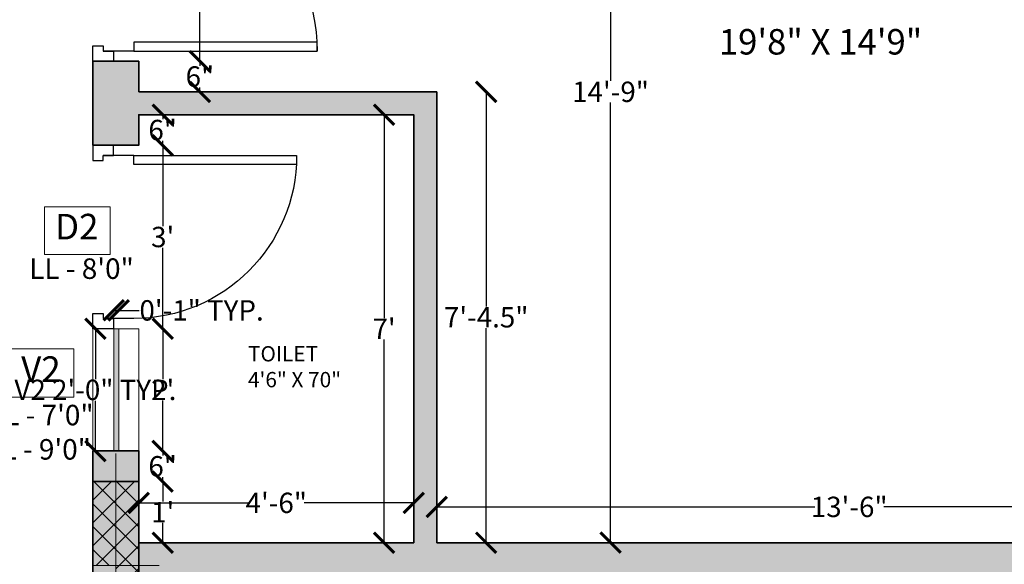
# Model space of a CAD drawing. Units: inches. Extents: x 2 to 905, y 9 to 678.
# Tile 4 of 8: x 102 to 295, y 367 to 474. Entities that reach past the tile are written whole.
import ezdxf

# ---------------------------------------------------------------- set-up
doc = ezdxf.new("R2010")
doc.units = ezdxf.units.IN
doc.linetypes.add('ACAD_ISO02W100', pattern=[15, 12, -3])
for name, color, linetype, lineweight in [('A-ANNO-DIMS', 7, 'Continuous', 18), ('A-COLS', 1, 'Continuous', 35), ('A-COLS-MARK', 1, 'Continuous', 18), ('A-COLS-PATT', 1, 'Continuous', 13), ('A-DOOR', 7, 'Continuous', 25), ('A-GLAZ', 4, 'Continuous', 18), ('A-WALL', 7, 'Continuous', 35), ('A-WALL-HIDN', 7, 'ACAD_ISO02W100', 18)]:
    doc.layers.add(name, color=color, linetype=linetype, lineweight=lineweight)
for name, color, linetype, lineweight, true_color in [('A-ANNO-IDEN', 251, 'Continuous', 18, 0x636466), ('A-AREA-IDEN', 252, 'Continuous', 18, 0x989898), ('A-WALL-PATT', 252, 'Continuous', 13, 0x939598)]:
    doc.layers.add(name, color=color, linetype=linetype, lineweight=lineweight, true_color=true_color)
doc.styles.add('PDF ArialMT', font='arial.ttf')
doc.styles.add('PDF Century Gothic Bold', font='txt')
doc.styles.get("Standard").update_dxf_attribs({"font": 'arial.ttf'})
doc.dimstyles.get("Standard").update_dxf_attribs({"dimtxt": 4, "dimasz": 4, "dimexe": 0.18, "dimexo": 0.0625, "dimgap": 0.09, "dimtad": 0, "dimtih": 1, "dimtoh": 1, "dimdec": 1, "dimzin": 0, "dimdsep": 46, "dimlunit": 3, "dimtxsty": 'Standard', "dimblk": 'ARCHTICK', "dimcen": 0, "dimse1": 1, "dimse2": 1, "dimclrt": 1, "dimadec": 0, "dimazin": 0, "dimtfac": 1, "dimtdec": 1, "dimtofl": 0, "dimtmove": 0, "dimatfit": 3, "dimfxl": 1, "dimtolj": 1, "dimtzin": 0, "dimarcsym": 0})

# ---------------------------------------------------------------- blocks, each defined once
blk = doc.blocks.new('*U4')
for p, q in [((0, 0), (0, -6)), ((-32, 0), (-32, -6))]:
    blk.add_line(p, q)
blk.add_lwpolyline([(0, 0), (0, 32), (-1.75, 32), (-1.75, 0)], close=True)
blk.add_arc((0, 0), 32, 90, 180)
blk = doc.blocks.new('*U5')
for p, q in [((0, 0), (0, -6)), ((36, 0), (36, -6))]:
    blk.add_line(p, q)
blk.add_lwpolyline([(0, 0), (0, 36), (1.75, 36), (1.75, 0)], close=True)
blk.add_arc((0, 0), 36, 0, 90)
blk = doc.blocks.new('_ArchTick')
at = {"color": 0, "linetype": 'ByBlock', "const_width": 0.15}
blk.add_lwpolyline([(-0.5, -0.5), (0.5, 0.5)], dxfattribs=at)
blk = doc.blocks.new('*D11')
at = {"layer": 'A-ANNO-DIMS', "color": 0, "lineweight": -2, "transparency": 16777216}
for p, q in [((218.07, 548.58), (218.07, 462.21)), ((218.07, 371.58), (218.07, 457.95))]:
    blk.add_line(p, q, dxfattribs=at)
at = {"layer": 'Defpoints', "color": 0, "transparency": 16777216}
for p in [(360.93, 548.58), (218.07, 371.58), (360.93, 371.58)]:
    blk.add_point(p, dxfattribs=at)
at = {"layer": 'A-ANNO-DIMS', "color": 0, "lineweight": -2, "transparency": 16777216, "xscale": 4, "yscale": 4, "zscale": 4}
for p, rotation in [((218.07, 548.58), 90), ((218.07, 371.58), 270)]:
    blk.add_blockref('_ArchTick', p, dxfattribs=dict(at, rotation=rotation))
at = {"layer": 'A-ANNO-DIMS', "color": 0, "transparency": 16777216, "insert": (218.07, 460.08), "char_height": 4, "attachment_point": 5}
blk.add_mtext('\\A1;14\'-9"', dxfattribs=at)
blk = doc.blocks.new('*D48')
at = {"layer": 'A-ANNO-DIMS', "color": 0, "lineweight": -2, "transparency": 16777216}
for p, q in [((130.12, 383.58), (130.12, 379.68)), ((130.12, 371.58), (130.12, 375.48))]:
    blk.add_line(p, q, dxfattribs=at)
at = {"layer": 'Defpoints', "color": 0, "transparency": 16777216}
for p in [(125.43, 383.58), (130.12, 383.58), (125.43, 371.58)]:
    blk.add_point(p, dxfattribs=at)
at = {"layer": 'A-ANNO-DIMS', "color": 0, "lineweight": -2, "transparency": 16777216, "xscale": 4, "yscale": 4, "zscale": 4}
for p, rotation in [((130.12, 383.58), 90), ((130.12, 371.58), 270)]:
    blk.add_blockref('_ArchTick', p, dxfattribs=dict(at, rotation=rotation))
at = {"layer": 'A-ANNO-DIMS', "color": 0, "transparency": 16777216, "insert": (130.12, 377.58), "char_height": 4, "attachment_point": 5}
blk.add_mtext("\\A1;1'", dxfattribs=at)
blk = doc.blocks.new('*D49')
at = {"layer": 'A-ANNO-DIMS', "color": 0, "lineweight": -2, "transparency": 16777216}
for p, q in [((130.12, 389.58), (130.12, 388.71)), ((130.12, 383.58), (130.12, 384.45))]:
    blk.add_line(p, q, dxfattribs=at)
at = {"layer": 'Defpoints', "color": 0, "transparency": 16777216}
for p in [(125.43, 389.58), (130.12, 389.58), (125.43, 383.58)]:
    blk.add_point(p, dxfattribs=at)
at = {"layer": 'A-ANNO-DIMS', "color": 0, "lineweight": -2, "transparency": 16777216, "xscale": 4, "yscale": 4, "zscale": 4}
for p, rotation in [((130.12, 389.58), 90), ((130.12, 383.58), 270)]:
    blk.add_blockref('_ArchTick', p, dxfattribs=dict(at, rotation=rotation))
at = {"layer": 'A-ANNO-DIMS', "color": 0, "transparency": 16777216, "insert": (130.12, 386.58), "char_height": 4, "attachment_point": 5}
blk.add_mtext('\\A1;6"', dxfattribs=at)
blk = doc.blocks.new('*D50')
at = {"layer": 'A-ANNO-DIMS', "color": 0, "lineweight": -2, "transparency": 16777216}
for p, q in [((130.12, 413.58), (130.12, 403.68)), ((130.12, 389.58), (130.12, 399.48))]:
    blk.add_line(p, q, dxfattribs=at)
at = {"layer": 'Defpoints', "color": 0, "transparency": 16777216}
for p in [(125.43, 413.58), (130.12, 413.58), (125.43, 389.58)]:
    blk.add_point(p, dxfattribs=at)
at = {"layer": 'A-ANNO-DIMS', "color": 0, "lineweight": -2, "transparency": 16777216, "xscale": 4, "yscale": 4, "zscale": 4}
for p, rotation in [((130.12, 413.58), 90), ((130.12, 389.58), 270)]:
    blk.add_blockref('_ArchTick', p, dxfattribs=dict(at, rotation=rotation))
at = {"layer": 'A-ANNO-DIMS', "color": 0, "transparency": 16777216, "insert": (130.12, 401.58), "char_height": 4, "attachment_point": 5}
blk.add_mtext("\\A1;2'", dxfattribs=at)
blk = doc.blocks.new('*D51')
at = {"layer": 'A-ANNO-DIMS', "color": 0, "lineweight": -2, "transparency": 16777216}
for p, q in [((130.12, 449.58), (130.12, 433.71)), ((130.12, 413.58), (130.12, 429.44))]:
    blk.add_line(p, q, dxfattribs=at)
at = {"layer": 'Defpoints', "color": 0, "transparency": 16777216}
for p in [(125.43, 449.58), (130.12, 449.58), (125.43, 413.58)]:
    blk.add_point(p, dxfattribs=at)
at = {"layer": 'A-ANNO-DIMS', "color": 0, "lineweight": -2, "transparency": 16777216, "xscale": 4, "yscale": 4, "zscale": 4}
for p, rotation in [((130.12, 449.58), 90), ((130.12, 413.58), 270)]:
    blk.add_blockref('_ArchTick', p, dxfattribs=dict(at, rotation=rotation))
at = {"layer": 'A-ANNO-DIMS', "color": 0, "transparency": 16777216, "insert": (130.12, 431.58), "char_height": 4, "attachment_point": 5}
blk.add_mtext("\\A1;3'", dxfattribs=at)
blk = doc.blocks.new('*D52')
at = {"layer": 'A-ANNO-DIMS', "color": 0, "lineweight": -2, "transparency": 16777216}
for p, q in [((130.12, 455.58), (130.12, 454.71)), ((130.12, 449.58), (130.12, 450.45))]:
    blk.add_line(p, q, dxfattribs=at)
at = {"layer": 'Defpoints', "color": 0, "transparency": 16777216}
for p in [(125.43, 455.58), (130.12, 455.58), (125.43, 449.58)]:
    blk.add_point(p, dxfattribs=at)
at = {"layer": 'A-ANNO-DIMS', "color": 0, "lineweight": -2, "transparency": 16777216, "xscale": 4, "yscale": 4, "zscale": 4}
for p, rotation in [((130.12, 455.58), 90), ((130.12, 449.58), 270)]:
    blk.add_blockref('_ArchTick', p, dxfattribs=dict(at, rotation=rotation))
at = {"layer": 'A-ANNO-DIMS', "color": 0, "transparency": 16777216, "insert": (130.12, 452.58), "char_height": 4, "attachment_point": 5}
blk.add_mtext('\\A1;6"', dxfattribs=at)
blk = doc.blocks.new('*D53')
at = {"layer": 'A-ANNO-DIMS', "color": 0, "lineweight": -2, "transparency": 16777216}
for p, q in [((137.43, 466.08), (137.43, 465.21)), ((137.43, 460.08), (137.43, 460.95))]:
    blk.add_line(p, q, dxfattribs=at)
at = {"layer": 'Defpoints', "color": 0, "transparency": 16777216}
for p in [(132.75, 466.08), (137.43, 466.08), (132.75, 460.08)]:
    blk.add_point(p, dxfattribs=at)
at = {"layer": 'A-ANNO-DIMS', "color": 0, "lineweight": -2, "transparency": 16777216, "xscale": 4, "yscale": 4, "zscale": 4}
for p, rotation in [((137.43, 466.08), 90), ((137.43, 460.08), 270)]:
    blk.add_blockref('_ArchTick', p, dxfattribs=dict(at, rotation=rotation))
at = {"layer": 'A-ANNO-DIMS', "color": 0, "transparency": 16777216, "insert": (137.43, 463.08), "char_height": 4, "attachment_point": 5}
blk.add_mtext('\\A1;6"', dxfattribs=at)
blk = doc.blocks.new('*D54')
at = {"layer": 'A-ANNO-DIMS', "color": 0, "lineweight": -2, "transparency": 16777216}
for p, q in [((137.43, 506.08), (137.43, 488.21)), ((137.43, 466.08), (137.43, 483.94))]:
    blk.add_line(p, q, dxfattribs=at)
at = {"layer": 'Defpoints', "color": 0, "transparency": 16777216}
for p in [(132.75, 506.08), (137.43, 506.08), (132.75, 466.08)]:
    blk.add_point(p, dxfattribs=at)
at = {"layer": 'A-ANNO-DIMS', "color": 0, "lineweight": -2, "transparency": 16777216, "xscale": 4, "yscale": 4, "zscale": 4}
for p, rotation in [((137.43, 506.08), 90), ((137.43, 466.08), 270)]:
    blk.add_blockref('_ArchTick', p, dxfattribs=dict(at, rotation=rotation))
at = {"layer": 'A-ANNO-DIMS', "color": 0, "transparency": 16777216, "insert": (137.43, 486.08), "char_height": 4, "attachment_point": 5}
blk.add_mtext('\\A1;3\'-4"', dxfattribs=at)
blk = doc.blocks.new('*D65')
at = {"layer": 'A-ANNO-DIMS', "color": 0, "lineweight": -2, "transparency": 16777216}
for p, q in [((183.93, 378.61), (258.16, 378.61)), ((345.93, 378.61), (271.71, 378.61))]:
    blk.add_line(p, q, dxfattribs=at)
at = {"layer": 'Defpoints', "color": 0, "transparency": 16777216}
for p in [(183.93, 378.61), (183.93, 371.58), (345.93, 371.58)]:
    blk.add_point(p, dxfattribs=at)
at = {"layer": 'A-ANNO-DIMS', "color": 0, "lineweight": -2, "transparency": 16777216, "xscale": 4, "yscale": 4, "zscale": 4, "rotation": 180}
blk.add_blockref('_ArchTick', (183.93, 378.61), dxfattribs=at)
at = {"layer": 'A-ANNO-DIMS', "color": 0, "lineweight": -2, "transparency": 16777216, "xscale": 4, "yscale": 4, "zscale": 4}
blk.add_blockref('_ArchTick', (345.93, 378.61), dxfattribs=at)
at = {"layer": 'A-ANNO-DIMS', "color": 0, "transparency": 16777216, "insert": (264.93, 378.61), "char_height": 4, "attachment_point": 5}
blk.add_mtext('\\A1;13\'-6"', dxfattribs=at)
blk = doc.blocks.new('*D66')
at = {"layer": 'A-ANNO-DIMS', "color": 0, "lineweight": -2, "transparency": 16777216}
for p, q in [((193.65, 460.08), (193.65, 417.95)), ((193.65, 371.58), (193.65, 413.7))]:
    blk.add_line(p, q, dxfattribs=at)
at = {"layer": 'Defpoints', "color": 0, "transparency": 16777216}
for p in [(183.93, 460.08), (193.65, 460.08), (183.93, 371.58)]:
    blk.add_point(p, dxfattribs=at)
at = {"layer": 'A-ANNO-DIMS', "color": 0, "lineweight": -2, "transparency": 16777216, "xscale": 4, "yscale": 4, "zscale": 4}
for p, rotation in [((193.65, 460.08), 90), ((193.65, 371.58), 270)]:
    blk.add_blockref('_ArchTick', p, dxfattribs=dict(at, rotation=rotation))
at = {"layer": 'A-ANNO-DIMS', "color": 0, "transparency": 16777216, "insert": (193.65, 415.83), "char_height": 4, "attachment_point": 5}
blk.add_mtext('\\A1;7\'-4.5"', dxfattribs=at)
blk = doc.blocks.new('*D83')
at = {"layer": 'A-ANNO-DIMS', "color": 0, "lineweight": -2, "transparency": 16777216}
for p, q in [((173.59, 455.58), (173.59, 415.67)), ((173.59, 371.58), (173.59, 411.49))]:
    blk.add_line(p, q, dxfattribs=at)
at = {"layer": 'Defpoints', "color": 0, "transparency": 16777216}
for p in [(173.59, 455.58), (179.43, 455.58), (179.43, 371.58)]:
    blk.add_point(p, dxfattribs=at)
at = {"layer": 'A-ANNO-DIMS', "color": 0, "lineweight": -2, "transparency": 16777216, "xscale": 4, "yscale": 4, "zscale": 4}
for p, rotation in [((173.59, 455.58), 90), ((173.59, 371.58), 270)]:
    blk.add_blockref('_ArchTick', p, dxfattribs=dict(at, rotation=rotation))
at = {"layer": 'A-ANNO-DIMS', "color": 0, "transparency": 16777216, "insert": (173.59, 413.58), "char_height": 4, "attachment_point": 5}
blk.add_mtext("\\A1;7'", dxfattribs=at)
blk = doc.blocks.new('*D84')
at = {"layer": 'A-ANNO-DIMS', "color": 0, "lineweight": -2, "transparency": 16777216}
for p, q in [((125.43, 379.4), (146.95, 379.4)), ((179.43, 379.4), (157.92, 379.4))]:
    blk.add_line(p, q, dxfattribs=at)
at = {"layer": 'Defpoints', "color": 0, "transparency": 16777216}
for p in [(179.43, 379.4), (125.43, 371.58), (179.43, 371.58)]:
    blk.add_point(p, dxfattribs=at)
at = {"layer": 'A-ANNO-DIMS', "color": 0, "lineweight": -2, "transparency": 16777216, "xscale": 4, "yscale": 4, "zscale": 4, "rotation": 180}
blk.add_blockref('_ArchTick', (125.43, 379.4), dxfattribs=at)
at = {"layer": 'A-ANNO-DIMS', "color": 0, "lineweight": -2, "transparency": 16777216, "xscale": 4, "yscale": 4, "zscale": 4}
blk.add_blockref('_ArchTick', (179.43, 379.4), dxfattribs=at)
at = {"layer": 'A-ANNO-DIMS', "color": 0, "transparency": 16777216, "insert": (152.43, 379.4), "char_height": 4, "attachment_point": 5}
blk.add_mtext('\\A1;4\'-6"', dxfattribs=at)
blk = doc.blocks.new('COL-DATUM-L')
h = blk.add_hatch(color=256)
h.dxf.hatch_style = 1
h.paths.add_polyline_path([(4.5, 0), (4.5, 4.5), (0, 4.5), (0, 0)])
for p, q in [((4.5, 0), (4.5, 26.48)), ((0, 4.5), (13.01, 4.5))]:
    blk.add_line(p, q)
blk.add_lwpolyline([(4.5, 0), (0, 0), (0, 4.5), (4.5, 4.5)], close=True)
blk = doc.blocks.new('GLAZ-V2-24')
h = blk.add_hatch(color=256)
h.dxf.hatch_style = 1
h.paths.add_polyline_path([(0.97, 24), (0, 24), (0, 0), (0.97, 0)])
for p, q in [((0, 0), (0, 24)), ((0.97, 0), (0.97, 24))]:
    blk.add_line(p, q)
blk = doc.blocks.new('DOOR-JAMB-REBATED')
blk.add_lwpolyline([(0, 0), (2, 0), (2, 1), (4, 1), (4, 3), (0, 3)], close=True)
blk = doc.blocks.new('*D98')
at = {"layer": 'A-ANNO-DIMS', "color": 0, "lineweight": -2, "transparency": 16777216}
for p, q in [((116.91, 413.58), (116.91, 403.71)), ((116.91, 389.58), (116.91, 399.45))]:
    blk.add_line(p, q, dxfattribs=at)
at = {"layer": 'Defpoints', "color": 0, "transparency": 16777216}
for p in [(116.91, 413.58), (120.51, 413.58), (120.51, 389.58)]:
    blk.add_point(p, dxfattribs=at)
at = {"layer": 'A-ANNO-DIMS', "color": 0, "lineweight": -2, "transparency": 16777216, "xscale": 4, "yscale": 4, "zscale": 4}
for p, rotation in [((116.91, 413.58), 90), ((116.91, 389.58), 270)]:
    blk.add_blockref('_ArchTick', p, dxfattribs=dict(at, rotation=rotation))
at = {"layer": 'A-ANNO-DIMS', "color": 1, "transparency": 16777216, "insert": (116.91, 401.58), "char_height": 4, "attachment_point": 5}
blk.add_mtext('\\A1;V2 2\'-0" TYP.', dxfattribs=at)
blk = doc.blocks.new('*D99')
at = {"layer": 'A-ANNO-DIMS', "color": 0, "lineweight": -2, "transparency": 16777216}
for p, q in [((120.51, 417.18), (121.48, 417.18)), ((121.48, 417.18), (125.48, 417.18))]:
    blk.add_line(p, q, dxfattribs=at)
at = {"layer": 'Defpoints', "color": 0, "transparency": 16777216}
for p in [(121.48, 417.18), (120.51, 413.58), (121.48, 413.58)]:
    blk.add_point(p, dxfattribs=at)
at = {"layer": 'A-ANNO-DIMS', "color": 0, "lineweight": -2, "transparency": 16777216, "xscale": 4, "yscale": 4, "zscale": 4, "rotation": 180}
blk.add_blockref('_ArchTick', (120.51, 417.18), dxfattribs=at)
at = {"layer": 'A-ANNO-DIMS', "color": 0, "lineweight": -2, "transparency": 16777216, "xscale": 4, "yscale": 4, "zscale": 4}
blk.add_blockref('_ArchTick', (121.48, 417.18), dxfattribs=at)
at = {"layer": 'A-ANNO-DIMS', "color": 1, "transparency": 16777216, "insert": (137.76, 417.18), "char_height": 4, "attachment_point": 5}
blk.add_mtext('\\A1;0\'-1" TYP.', dxfattribs=at)
blk = doc.blocks.new('*D120')
at = {"layer": 'A-ANNO-DIMS', "color": 0, "lineweight": -2, "transparency": 16777216}
for p, q in [((179.43, 671.82), (183.93, 671.82)), ((183.93, 671.82), (187.93, 671.82))]:
    blk.add_line(p, q, dxfattribs=at)
at = {"layer": 'Defpoints', "color": 0, "transparency": 16777216}
for p in [(183.93, 671.82), (183.93, 460.08), (179.43, 455.58)]:
    blk.add_point(p, dxfattribs=at)
at = {"layer": 'A-ANNO-DIMS', "color": 0, "lineweight": -2, "transparency": 16777216, "xscale": 4, "yscale": 4, "zscale": 4, "rotation": 180}
blk.add_blockref('_ArchTick', (179.43, 671.82), dxfattribs=at)
at = {"layer": 'A-ANNO-DIMS', "color": 0, "lineweight": -2, "transparency": 16777216, "xscale": 4, "yscale": 4, "zscale": 4}
blk.add_blockref('_ArchTick', (183.93, 671.82), dxfattribs=at)
at = {"layer": 'A-ANNO-DIMS', "color": 1, "transparency": 16777216, "insert": (198, 671.82), "char_height": 4, "attachment_point": 5}
blk.add_mtext('\\A1;0\'-4 1/2"', dxfattribs=at)

msp = doc.modelspace()

# ---------------------------------------------------------------- hatches: boundary and pattern name
at = {"layer": 'A-COLS-PATT'}
h = msp.add_hatch(dxfattribs=at)
h.set_pattern_fill('ANSI37', color=256)
h.set_pattern_definition([(45, (895.109, 27.1098), (-2.245064, 2.245064), []), (135, (895.109, 27.1098), (-2.245064, -2.245064), [])])
h.paths.add_polyline_path([(125.43, 367.08), (120.93, 367.08), (120.93, 362.58), (125.43, 362.58)])
h.paths.add_polyline_path([(125.43, 383.58), (120.93, 383.58), (120.93, 367.08), (125.43, 367.08)])
h.paths.add_polyline_path([(120.93, 383.58), (116.43, 383.58), (116.43, 367.08), (120.93, 367.08)])
at = {"layer": 'A-WALL-PATT'}
h = msp.add_hatch(color=256, dxfattribs=at)
h.dxf.hatch_style = 1
h.paths.add_polyline_path([(125.43, 227.58), (116.43, 227.58), (116.43, 128.58), (237.93, 128.58), (237.93, 137.58), (125.43, 137.58)])
h.paths.add_polyline_path([(249.93, 302.58), (183.93, 302.58), (183.93, 320.58), (179.43, 320.58), (179.43, 302.58), (116.43, 302.58), (116.43, 275.58), (125.43, 275.58), (125.43, 293.58), (249.93, 293.58), (249.93, 297.58)], flags=0)
h.paths.add_polyline_path([(369.93, 137.58), (360.93, 137.58), (360.93, 218.58), (369.93, 218.58), (369.93, 227.58), (363.93, 227.58), (351.93, 227.58), (351.93, 137.58), (345.93, 137.58), (345.93, 128.58), (360.93, 128.58), (369.93, 128.58)])
h.paths.add_polyline_path([(297.93, 137.58), (285.93, 137.58), (285.93, 128.58), (297.93, 128.58)])
h.paths.add_polyline_path([(369.93, 444.58), (360.93, 444.58), (360.93, 371.58), (183.93, 371.58), (183.93, 460.08), (125.43, 460.08), (125.43, 466.08), (116.43, 466.08), (116.43, 449.58), (120.43, 449.58), (125.43, 449.58), (125.43, 455.58), (179.43, 455.58), (179.43, 371.58), (125.43, 371.58), (125.43, 389.58), (116.43, 389.58), (116.43, 362.58), (179.43, 362.58), (179.43, 344.58), (183.93, 344.58), (183.93, 362.58), (291.93, 362.58), (291.93, 302.58), (285.93, 302.58), (285.93, 293.58), (309.93, 293.58), (309.93, 302.58), (300.93, 302.58), (300.93, 362.58), (360.93, 362.58), (360.93, 302.58), (351.93, 302.58), (351.93, 293.58), (360.93, 293.58), (360.93, 275.58), (363.93, 275.58), (369.93, 275.58)])
h.paths.add_polyline_path([(282.93, 557.58), (116.43, 557.58), (116.43, 506.08), (120.43, 506.08), (125.43, 506.08), (125.43, 548.58), (282.93, 548.58)])
h.paths.add_polyline_path([(369.93, 557.58), (330.93, 557.58), (330.93, 548.58), (360.93, 548.58), (360.93, 504.58), (369.93, 504.58)])

# ---------------------------------------------------------------- linework, layer by layer
at = {"layer": 'A-ANNO-IDEN'}
for points in [[(106.88, 437.5), (119.78, 437.5), (119.78, 428.13), (106.88, 428.13)], [(99.78, 409.64), (112.68, 409.64), (112.68, 400.16), (99.78, 400.16)]]:
    msp.add_lwpolyline(points, close=True, dxfattribs=at)
at = {"layer": 'A-COLS'}
msp.add_lwpolyline([(116.43, 383.58), (125.43, 383.58), (125.43, 362.58), (116.43, 362.58)], close=True, dxfattribs=at)
at = {"layer": 'A-GLAZ'}
msp.add_lwpolyline([(116.43, 389.58), (116.43, 413.58), (125.43, 413.58), (125.43, 389.58)], close=True, dxfattribs=at)
at = {"layer": 'A-WALL'}
for p, q in [((125.43, 466.08), (116.43, 466.08)), ((116.43, 466.08), (116.43, 449.58)), ((125.43, 466.08), (125.43, 460.08)), ((183.93, 460.08), (125.43, 460.08)), ((183.93, 371.58), (183.93, 460.08)), ((125.43, 389.58), (116.43, 389.58)), ((116.43, 389.58), (116.43, 362.58)), ((183.93, 371.58), (360.93, 371.58))]:
    msp.add_line(p, q, dxfattribs=at)
msp.add_lwpolyline([(125.43, 389.58), (125.43, 371.58), (179.43, 371.58), (179.43, 455.58), (125.43, 455.58), (125.43, 449.58), (116.43, 449.58)], dxfattribs=at)
at = {"layer": 'A-WALL-HIDN'}
msp.add_line((120.93, 389.58), (125.43, 389.58), dxfattribs=at)
msp.add_lwpolyline([(120.93, 413.58), (125.43, 413.58), (116.43, 413.58)], dxfattribs=at)

# ---------------------------------------------------------------- block references
at = {"layer": 'A-COLS-MARK'}
msp.add_blockref('COL-DATUM-L', (116.43, 362.58), dxfattribs=at)
at = {"layer": 'A-DOOR', "xscale": -1, "rotation": 270}
for name, p in [('*U5', (124.43, 468.08)), ('*U4', (124.43, 447.58))]:
    msp.add_blockref(name, p, dxfattribs=at)
at = {"layer": 'A-DOOR', "extrusion": (0, 0, -1), "zscale": -1, "rotation": 180}
for p in [(-116.43, 469.08), (-116.43, 416.58)]:
    msp.add_blockref('DOOR-JAMB-REBATED', p, dxfattribs=at)
at = {"layer": 'A-DOOR'}
msp.add_blockref('DOOR-JAMB-REBATED', (116.43, 446.58), dxfattribs=at)
at = {"layer": 'A-GLAZ'}
msp.add_blockref('GLAZ-V2-24', (120.51, 389.58), dxfattribs=at)

# ---------------------------------------------------------------- texts
at = {"layer": 'A-ANNO-IDEN', "attachment_point": 4, "style": 'PDF ArialMT'}
for s, insert, char_height in [('D2', (108.98, 432.96), 5.029), ('LL - 8\'0"', (103.91, 424.85), 4.023), ('V2', (102.33, 404.99), 5.029), ('SL - 7\'0"', (95.72, 396.11), 4.023), ('LL - 9\'0"', (95.49, 389.38), 4.023)]:
    msp.add_mtext(s, dxfattribs=dict(at, insert=insert, char_height=char_height))
at = {"layer": 'A-AREA-IDEN', "attachment_point": 4, "style": 'PDF Century Gothic Bold'}
for s, insert, char_height in [('19\'8" X 14\'9"', (239.34, 469.25), 5), ('TOILET', (146.87, 408.27), 3), ('4\'6" X 70"', (146.87, 403.2), 3)]:
    msp.add_mtext(s, dxfattribs=dict(at, insert=insert, char_height=char_height))

# ---------------------------------------------------------------- dimensions: what is measured, and where the dimension line sits
at = {"layer": 'A-ANNO-DIMS'}
for base, p1, p2, override, picture, middle in [((183.93, 671.82), (179.43, 455.58), (183.93, 460.08), {"dimdec": 1, "dimlfac": 1, "dimrnd": 0, "dimzin": 1, "dimdsep": 46, "dimlunit": 4, "dimfrac": 2}, '*D120', (198, 671.82)), ((179.43, 379.4), (125.43, 371.58), (179.43, 371.58), {"dimdec": 0, "dimclrd": 0, "dimclre": 0, "dimclrt": 0}, '*D84', (152.43, 379.4)), ((183.93, 378.61), (345.93, 371.58), (183.93, 371.58), {"dimdec": 0, "dimclrd": 0, "dimclre": 0, "dimclrt": 0, "dimtmove": 1}, '*D65', (264.93, 378.61))]:
    dim = msp.add_linear_dim(base=base, p1=p1, p2=p2, dimstyle='Standard', override=override, dxfattribs=at)
    dim.commit()
    dim.dimension.update_dxf_attribs({"geometry": picture, "text_midpoint": middle})
for base, p1, p2, override, picture, middle in [((218.07, 371.58), (360.93, 548.58), (360.93, 371.58), {"dimdec": 0, "dimclrd": 0, "dimclre": 0, "dimclrt": 0}, '*D11', (218.07, 460.08)), ((137.43, 506.08), (132.75, 466.08), (132.75, 506.08), {"dimdec": 0, "dimclrd": 0, "dimclre": 0, "dimclrt": 0, "dimtmove": 1}, '*D54', (137.43, 486.08)), ((137.43, 466.08), (132.75, 460.08), (132.75, 466.08), {"dimdec": 0, "dimclrd": 0, "dimclre": 0, "dimclrt": 0}, '*D53', (137.43, 463.08)), ((193.65, 460.08), (183.93, 371.58), (183.93, 460.08), {"dimclrd": 0, "dimclre": 0, "dimclrt": 0}, '*D66', (193.65, 415.83)), ((130.12, 455.58), (125.43, 449.58), (125.43, 455.58), {"dimdec": 0, "dimclrd": 0, "dimclre": 0, "dimclrt": 0, "dimtmove": 1}, '*D52', (130.12, 452.58)), ((173.59, 455.58), (179.43, 371.58), (179.43, 455.58), {"dimclrd": 0, "dimclre": 0, "dimclrt": 0}, '*D83', (173.59, 413.58)), ((130.12, 449.58), (125.43, 413.58), (125.43, 449.58), {"dimclrd": 0, "dimclre": 0, "dimclrt": 0, "dimtmove": 1}, '*D51', (130.12, 431.58)), ((130.12, 413.58), (125.43, 389.58), (125.43, 413.58), {"dimclrd": 0, "dimclre": 0, "dimclrt": 0, "dimtmove": 1}, '*D50', (130.12, 401.58)), ((130.12, 389.58), (125.43, 383.58), (125.43, 389.58), {"dimdec": 0, "dimclrd": 0, "dimclre": 0, "dimclrt": 0, "dimtmove": 1}, '*D49', (130.12, 386.58)), ((130.12, 383.58), (125.43, 371.58), (125.43, 383.58), {"dimclrd": 0, "dimclre": 0, "dimclrt": 0}, '*D48', (130.12, 377.58))]:
    dim = msp.add_linear_dim(base=base, p1=p1, p2=p2, angle=90, dimstyle='Standard', override=override, dxfattribs=at)
    dim.commit()
    dim.dimension.update_dxf_attribs({"geometry": picture, "text_midpoint": middle})
dim = msp.add_linear_dim(base=(121.48, 417.18), p1=(120.51, 413.58), p2=(121.48, 413.58), text='<> TYP.', dimstyle='Standard', override={"dimdec": 1, "dimlfac": 1, "dimrnd": 0, "dimzin": 1, "dimdsep": 46, "dimlunit": 4, "dimfrac": 2}, dxfattribs=at)
dim.commit()
dim.dimension.update_dxf_attribs({"geometry": '*D99', "text_midpoint": (137.76, 417.18)})
dim = msp.add_linear_dim(base=(116.91, 413.58), p1=(120.51, 389.58), p2=(120.51, 413.58), angle=90, text='V2 <> TYP.', dimstyle='Standard', override={"dimdec": 1, "dimlfac": 1, "dimrnd": 0, "dimzin": 1, "dimdsep": 46, "dimlunit": 4, "dimfrac": 2}, dxfattribs=at)
dim.commit()
dim.dimension.update_dxf_attribs({"geometry": '*D98', "text_midpoint": (116.91, 401.58)})

doc.saveas('drawing.dxf')
